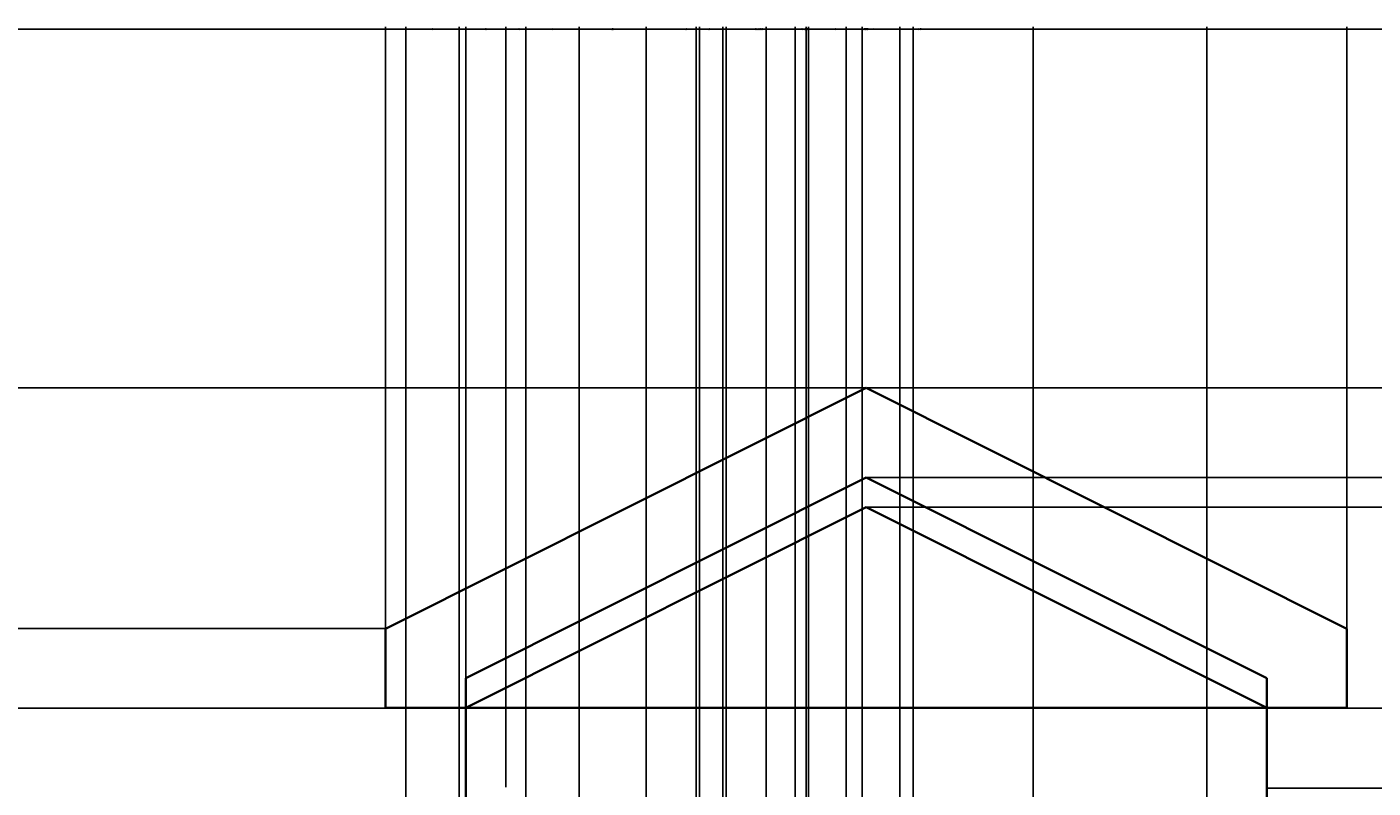
# Model space of a CAD drawing. Units: inches. Extents: x 2154 to 2740, y 571 to 1084.
# Tile 11 of 13: x 2384 to 2485, y 1027 to 1084. Entities that reach past the tile are written whole.
import ezdxf

# ---------------------------------------------------------------- set-up
doc = ezdxf.new("R2010")
doc.units = ezdxf.units.IN
doc.layers.add('A-ANNO-DIMS', color=2, linetype='Continuous', lineweight=18)
doc.layers.add('A-ROOF', color=1, linetype='Continuous', lineweight=35)
doc.styles.get("Standard").update_dxf_attribs({"font": 'arial.ttf'})
doc.dimstyles.get("Standard").update_dxf_attribs({"dimtxt": 0.18, "dimasz": 0.18, "dimexe": 0.18, "dimexo": 0.0625, "dimgap": 0.09, "dimtad": 0, "dimtih": 1, "dimtoh": 1, "dimdec": 4, "dimzin": 0, "dimdsep": 46, "dimtxsty": 'Standard', "dimcen": 0.09, "dimadec": 0, "dimazin": 0, "dimtfac": 1, "dimtdec": 4, "dimtofl": 0, "dimtmove": 0, "dimatfit": 3, "dimfxl": 1, "dimtolj": 1, "dimtzin": 0, "dimarcsym": 0})

# ---------------------------------------------------------------- blocks, each defined once
blk = doc.blocks.new('*D7')
at = {"layer": 'A-ANNO-DIMS', "color": 0, "lineweight": -2, "transparency": 16777216}
for p, q in [((2181.21, 981.59), (2181.21, 1084.04)), ((2181.39, 1083.86), (2446.92, 1083.86)), ((2713.03, 1083.86), (2447.49, 1083.86)), ((2713.21, 981.59), (2713.21, 1084.04))]:
    blk.add_line(p, q, dxfattribs=at)
at = {"layer": 'A-ANNO-DIMS', "color": 0, "transparency": 16777216}
for points in [[(2181.39, 1083.89), (2181.39, 1083.83), (2181.21, 1083.86)], [(2713.03, 1083.89), (2713.03, 1083.83), (2713.21, 1083.86)]]:
    blk.add_solid(points, dxfattribs=at)
at = {"layer": 'Defpoints', "color": 0, "transparency": 16777216}
for p in [(2713.21, 1083.86), (2181.21, 981.53), (2713.21, 981.53)]:
    blk.add_point(p, dxfattribs=at)
at = {"layer": 'A-ANNO-DIMS', "color": 0, "transparency": 16777216, "insert": (2447.21, 1083.86), "char_height": 0.18, "attachment_point": 5}
blk.add_mtext('\\A1;532', dxfattribs=at)
blk = doc.blocks.new('*D10')
at = {"layer": 'A-ANNO-DIMS', "color": 0, "lineweight": -2, "transparency": 16777216}
for p, q in [((2447.14, 1057.01), (2154.18, 1057.01)), ((2154.36, 1056.83), (2154.36, 827.45)), ((2154.36, 597.71), (2154.36, 827.09)), ((2181.14, 597.53), (2154.18, 597.53))]:
    blk.add_line(p, q, dxfattribs=at)
at = {"layer": 'A-ANNO-DIMS', "color": 0, "transparency": 16777216}
for points in [[(2154.33, 1056.83), (2154.39, 1056.83), (2154.36, 1057.01)], [(2154.33, 597.71), (2154.39, 597.71), (2154.36, 597.53)]]:
    blk.add_solid(points, dxfattribs=at)
at = {"layer": 'Defpoints', "color": 0, "transparency": 16777216}
for p in [(2154.36, 1057.01), (2447.21, 1057.01), (2181.21, 597.53)]:
    blk.add_point(p, dxfattribs=at)
at = {"layer": 'A-ANNO-DIMS', "color": 0, "transparency": 16777216, "insert": (2154.36, 827.27), "char_height": 0.18, "attachment_point": 5}
blk.add_mtext('\\A1;459.5', dxfattribs=at)
blk = doc.blocks.new('*D13')
at = {"layer": 'A-ANNO-DIMS', "color": 0, "lineweight": -2, "transparency": 16777216}
for p, q in [((2447.27, 1057.01), (2740.24, 1057.01)), ((2740.06, 1056.83), (2740.06, 1019.45)), ((2740.06, 981.71), (2740.06, 1019.09)), ((2713.27, 981.53), (2740.24, 981.53))]:
    blk.add_line(p, q, dxfattribs=at)
at = {"layer": 'A-ANNO-DIMS', "color": 0, "transparency": 16777216}
for points in [[(2740.03, 1056.83), (2740.09, 1056.83), (2740.06, 1057.01)], [(2740.03, 981.71), (2740.09, 981.71), (2740.06, 981.53)]]:
    blk.add_solid(points, dxfattribs=at)
at = {"layer": 'Defpoints', "color": 0, "transparency": 16777216}
for p in [(2447.21, 1057.01), (2740.06, 1057.01), (2713.21, 981.53)]:
    blk.add_point(p, dxfattribs=at)
at = {"layer": 'A-ANNO-DIMS', "color": 0, "transparency": 16777216, "insert": (2740.06, 1019.27), "char_height": 0.18, "attachment_point": 5}
blk.add_mtext('\\A1;75.47', dxfattribs=at)
blk = doc.blocks.new('*D32')
at = {"layer": 'A-ANNO-DIMS', "color": 0, "lineweight": -2, "transparency": 16777216}
for p, q in [((2412.71, 873.59), (2412.71, 1084.04)), ((2412.89, 1083.86), (2442.49, 1083.86)), ((2472.53, 1083.86), (2442.93, 1083.86)), ((2472.71, 873.59), (2472.71, 1084.04))]:
    blk.add_line(p, q, dxfattribs=at)
at = {"layer": 'A-ANNO-DIMS', "color": 0, "transparency": 16777216}
for points in [[(2412.89, 1083.89), (2412.89, 1083.83), (2412.71, 1083.86)], [(2472.53, 1083.89), (2472.53, 1083.83), (2472.71, 1083.86)]]:
    blk.add_solid(points, dxfattribs=at)
at = {"layer": 'Defpoints', "color": 0, "transparency": 16777216}
for p in [(2472.71, 1083.86), (2412.71, 873.53), (2472.71, 873.53)]:
    blk.add_point(p, dxfattribs=at)
at = {"layer": 'A-ANNO-DIMS', "color": 0, "transparency": 16777216, "insert": (2442.71, 1083.86), "char_height": 0.18, "attachment_point": 5}
blk.add_mtext('\\A1;60', dxfattribs=at)
blk = doc.blocks.new('*D34')
at = {"layer": 'A-ANNO-DIMS', "color": 0, "lineweight": -2, "transparency": 16777216}
for p, q in [((2417.14, 1033.01), (2154.18, 1033.01)), ((2154.36, 1032.83), (2154.36, 1001.96)), ((2154.36, 970.71), (2154.36, 1001.59)), ((2417.14, 970.53), (2154.18, 970.53))]:
    blk.add_line(p, q, dxfattribs=at)
at = {"layer": 'A-ANNO-DIMS', "color": 0, "transparency": 16777216}
for points in [[(2154.33, 1032.83), (2154.39, 1032.83), (2154.36, 1033.01)], [(2154.33, 970.71), (2154.39, 970.71), (2154.36, 970.53)]]:
    blk.add_solid(points, dxfattribs=at)
at = {"layer": 'Defpoints', "color": 0, "transparency": 16777216}
for p in [(2154.36, 1033.01), (2417.21, 1033.01), (2417.21, 970.53)]:
    blk.add_point(p, dxfattribs=at)
at = {"layer": 'A-ANNO-DIMS', "color": 0, "transparency": 16777216, "insert": (2154.36, 1001.77), "char_height": 0.18, "attachment_point": 5}
blk.add_mtext('\\A1;62.48', dxfattribs=at)
blk = doc.blocks.new('*D66')
at = {"layer": 'A-ANNO-DIMS', "color": 0, "lineweight": -2, "transparency": 16777216}
for p, q in [((2411.21, 1033.08), (2411.21, 1084.04)), ((2411.39, 1083.86), (2446.99, 1083.86)), ((2483.03, 1083.86), (2447.42, 1083.86)), ((2483.21, 1033.08), (2483.21, 1084.04))]:
    blk.add_line(p, q, dxfattribs=at)
at = {"layer": 'A-ANNO-DIMS', "color": 0, "transparency": 16777216}
for points in [[(2411.39, 1083.89), (2411.39, 1083.83), (2411.21, 1083.86)], [(2483.03, 1083.89), (2483.03, 1083.83), (2483.21, 1083.86)]]:
    blk.add_solid(points, dxfattribs=at)
at = {"layer": 'Defpoints', "color": 0, "transparency": 16777216}
for p in [(2483.21, 1083.86), (2411.21, 1033.01), (2483.21, 1033.01)]:
    blk.add_point(p, dxfattribs=at)
at = {"layer": 'A-ANNO-DIMS', "color": 0, "transparency": 16777216, "insert": (2447.21, 1083.86), "char_height": 0.18, "attachment_point": 5}
blk.add_mtext('\\A1;72', dxfattribs=at)
blk = doc.blocks.new('*D67')
at = {"layer": 'A-ANNO-DIMS', "color": 0, "lineweight": -2, "transparency": 16777216}
for p, q in [((2411.14, 1038.96), (2154.18, 1038.96)), ((2154.36, 1038.78), (2154.36, 1036.17)), ((2154.36, 1033.19), (2154.36, 1035.8)), ((2411.14, 1033.01), (2154.18, 1033.01))]:
    blk.add_line(p, q, dxfattribs=at)
at = {"layer": 'A-ANNO-DIMS', "color": 0, "transparency": 16777216}
for points in [[(2154.33, 1038.78), (2154.39, 1038.78), (2154.36, 1038.96)], [(2154.33, 1033.19), (2154.39, 1033.19), (2154.36, 1033.01)]]:
    blk.add_solid(points, dxfattribs=at)
at = {"layer": 'Defpoints', "color": 0, "transparency": 16777216}
for p in [(2154.36, 1038.96), (2411.21, 1038.96), (2411.21, 1033.01)]:
    blk.add_point(p, dxfattribs=at)
at = {"layer": 'A-ANNO-DIMS', "color": 0, "transparency": 16777216, "insert": (2154.36, 1035.99), "char_height": 0.18, "attachment_point": 5}
blk.add_mtext('\\A1;5.941', dxfattribs=at)
blk = doc.blocks.new('*D68')
at = {"layer": 'A-ANNO-DIMS', "color": 0, "lineweight": -2, "transparency": 16777216}
for p, q in [((2447.14, 1057.01), (2154.18, 1057.01)), ((2154.36, 1056.83), (2154.36, 1048.16)), ((2154.36, 1039.14), (2154.36, 1047.8)), ((2411.14, 1038.96), (2154.18, 1038.96))]:
    blk.add_line(p, q, dxfattribs=at)
at = {"layer": 'A-ANNO-DIMS', "color": 0, "transparency": 16777216}
for points in [[(2154.33, 1056.83), (2154.39, 1056.83), (2154.36, 1057.01)], [(2154.33, 1039.14), (2154.39, 1039.14), (2154.36, 1038.96)]]:
    blk.add_solid(points, dxfattribs=at)
at = {"layer": 'Defpoints', "color": 0, "transparency": 16777216}
for p in [(2154.36, 1057.01), (2447.21, 1057.01), (2411.21, 1038.96)]:
    blk.add_point(p, dxfattribs=at)
at = {"layer": 'A-ANNO-DIMS', "color": 0, "transparency": 16777216, "insert": (2154.36, 1047.98), "char_height": 0.18, "attachment_point": 5}
blk.add_mtext('\\A1;18.05', dxfattribs=at)
blk = doc.blocks.new('*D69')
at = {"layer": 'A-ANNO-DIMS', "color": 0, "lineweight": -2, "transparency": 16777216}
for p, q in [((2447.27, 1057.01), (2740.24, 1057.01)), ((2740.06, 1056.83), (2740.06, 1053.83)), ((2740.06, 1050.47), (2740.06, 1053.47)), ((2447.27, 1050.29), (2740.24, 1050.29))]:
    blk.add_line(p, q, dxfattribs=at)
at = {"layer": 'A-ANNO-DIMS', "color": 0, "transparency": 16777216}
for points in [[(2740.03, 1056.83), (2740.09, 1056.83), (2740.06, 1057.01)], [(2740.03, 1050.47), (2740.09, 1050.47), (2740.06, 1050.29)]]:
    blk.add_solid(points, dxfattribs=at)
at = {"layer": 'Defpoints', "color": 0, "transparency": 16777216}
for p in [(2447.21, 1057.01), (2740.06, 1057.01), (2447.21, 1050.29)]:
    blk.add_point(p, dxfattribs=at)
at = {"layer": 'A-ANNO-DIMS', "color": 0, "transparency": 16777216, "insert": (2740.06, 1053.65), "char_height": 0.18, "attachment_point": 5}
blk.add_mtext('\\A1;6.712', dxfattribs=at)
blk = doc.blocks.new('*D70')
at = {"layer": 'A-ANNO-DIMS', "color": 0, "lineweight": -2, "transparency": 16777216}
for p, q in [((2447.27, 1050.29), (2740.24, 1050.29)), ((2740.06, 1050.11), (2740.06, 1049.36)), ((2740.06, 1048.24), (2740.06, 1048.99)), ((2447.27, 1048.06), (2740.24, 1048.06))]:
    blk.add_line(p, q, dxfattribs=at)
at = {"layer": 'A-ANNO-DIMS', "color": 0, "transparency": 16777216}
for points in [[(2740.03, 1050.11), (2740.09, 1050.11), (2740.06, 1050.29)], [(2740.03, 1048.24), (2740.09, 1048.24), (2740.06, 1048.06)]]:
    blk.add_solid(points, dxfattribs=at)
at = {"layer": 'Defpoints', "color": 0, "transparency": 16777216}
for p in [(2447.21, 1050.29), (2740.06, 1050.29), (2447.21, 1048.06)]:
    blk.add_point(p, dxfattribs=at)
at = {"layer": 'A-ANNO-DIMS', "color": 0, "transparency": 16777216, "insert": (2740.06, 1049.17), "char_height": 0.18, "attachment_point": 5}
blk.add_mtext('\\A1;2.24', dxfattribs=at)
blk = doc.blocks.new('*D71')
at = {"layer": 'A-ANNO-DIMS', "color": 0, "lineweight": -2, "transparency": 16777216}
for p, q in [((2477.27, 1033.01), (2740.24, 1033.01)), ((2740.06, 1032.83), (2740.06, 1030.2)), ((2740.06, 1027.19), (2740.06, 1029.83)), ((2477.27, 1027.01), (2740.24, 1027.01))]:
    blk.add_line(p, q, dxfattribs=at)
at = {"layer": 'A-ANNO-DIMS', "color": 0, "transparency": 16777216}
for points in [[(2740.03, 1032.83), (2740.09, 1032.83), (2740.06, 1033.01)], [(2740.03, 1027.19), (2740.09, 1027.19), (2740.06, 1027.01)]]:
    blk.add_solid(points, dxfattribs=at)
at = {"layer": 'Defpoints', "color": 0, "transparency": 16777216}
for p in [(2477.21, 1033.01), (2740.06, 1033.01), (2477.21, 1027.01)]:
    blk.add_point(p, dxfattribs=at)
at = {"layer": 'A-ANNO-DIMS', "color": 0, "transparency": 16777216, "insert": (2740.06, 1030.01), "char_height": 0.18, "attachment_point": 5}
blk.add_mtext('\\A1;6', dxfattribs=at)
blk = doc.blocks.new('*D72')
at = {"layer": 'A-ANNO-DIMS', "color": 0, "lineweight": -2, "transparency": 16777216}
for p, q in [((2477.27, 1027.01), (2740.24, 1027.01)), ((2740.06, 1026.83), (2740.06, 1001.96)), ((2740.06, 976.71), (2740.06, 1001.59)), ((2477.27, 976.53), (2740.24, 976.53))]:
    blk.add_line(p, q, dxfattribs=at)
at = {"layer": 'A-ANNO-DIMS', "color": 0, "transparency": 16777216}
for points in [[(2740.03, 1026.83), (2740.09, 1026.83), (2740.06, 1027.01)], [(2740.03, 976.71), (2740.09, 976.71), (2740.06, 976.53)]]:
    blk.add_solid(points, dxfattribs=at)
at = {"layer": 'Defpoints', "color": 0, "transparency": 16777216}
for p in [(2477.21, 1027.01), (2740.06, 1027.01), (2477.21, 976.53)]:
    blk.add_point(p, dxfattribs=at)
at = {"layer": 'A-ANNO-DIMS', "color": 0, "transparency": 16777216, "insert": (2740.06, 1001.77), "char_height": 0.18, "attachment_point": 5}
blk.add_mtext('\\A1;50.48', dxfattribs=at)
blk = doc.blocks.new('*D74')
at = {"layer": 'A-ANNO-DIMS', "color": 0, "lineweight": -2, "transparency": 16777216}
for p, q in [((2417.21, 1027.08), (2417.21, 1084.04)), ((2417.39, 1083.86), (2418.56, 1083.86)), ((2420.03, 1083.86), (2418.86, 1083.86)), ((2420.21, 1027.08), (2420.21, 1084.04))]:
    blk.add_line(p, q, dxfattribs=at)
at = {"layer": 'A-ANNO-DIMS', "color": 0, "transparency": 16777216}
for points in [[(2417.39, 1083.89), (2417.39, 1083.83), (2417.21, 1083.86)], [(2420.03, 1083.89), (2420.03, 1083.83), (2420.21, 1083.86)]]:
    blk.add_solid(points, dxfattribs=at)
at = {"layer": 'Defpoints', "color": 0, "transparency": 16777216}
for p in [(2420.21, 1083.86), (2417.21, 1027.01), (2420.21, 1027.01)]:
    blk.add_point(p, dxfattribs=at)
at = {"layer": 'A-ANNO-DIMS', "color": 0, "transparency": 16777216, "insert": (2418.71, 1083.86), "char_height": 0.18, "attachment_point": 5}
blk.add_mtext('\\A1;3', dxfattribs=at)
blk = doc.blocks.new('*D79')
at = {"layer": 'A-ANNO-DIMS', "color": 0, "lineweight": -2, "transparency": 16777216}
for p, q in [((2436.46, 1010.97), (2436.46, 1084.04)), ((2436.64, 1083.86), (2438.78, 1083.86)), ((2441.71, 1083.86), (2439.57, 1083.86)), ((2441.89, 1010.97), (2441.89, 1084.04))]:
    blk.add_line(p, q, dxfattribs=at)
at = {"layer": 'A-ANNO-DIMS', "color": 0, "transparency": 16777216}
for points in [[(2436.64, 1083.89), (2436.64, 1083.83), (2436.46, 1083.86)], [(2441.71, 1083.89), (2441.71, 1083.83), (2441.89, 1083.86)]]:
    blk.add_solid(points, dxfattribs=at)
at = {"layer": 'Defpoints', "color": 0, "transparency": 16777216}
for p in [(2441.89, 1083.86), (2436.46, 1010.91), (2441.89, 1010.91)]:
    blk.add_point(p, dxfattribs=at)
at = {"layer": 'A-ANNO-DIMS', "color": 0, "transparency": 16777216, "insert": (2439.17, 1083.86), "char_height": 0.18, "attachment_point": 5}
blk.add_mtext('\\A1;5.433', dxfattribs=at)
blk = doc.blocks.new('*D80')
at = {"layer": 'A-ANNO-DIMS', "color": 0, "lineweight": -2, "transparency": 16777216}
for p, q in [((2441.89, 1010.97), (2441.89, 1084.04)), ((2442.07, 1083.86), (2442.27, 1083.86)), ((2442.71, 1083.86), (2442.51, 1083.86)), ((2442.89, 1010.97), (2442.89, 1084.04))]:
    blk.add_line(p, q, dxfattribs=at)
at = {"layer": 'A-ANNO-DIMS', "color": 0, "transparency": 16777216}
for points in [[(2442.07, 1083.89), (2442.07, 1083.83), (2441.89, 1083.86)], [(2442.71, 1083.89), (2442.71, 1083.83), (2442.89, 1083.86)]]:
    blk.add_solid(points, dxfattribs=at)
at = {"layer": 'Defpoints', "color": 0, "transparency": 16777216}
for p in [(2442.89, 1083.86), (2441.89, 1010.91), (2442.89, 1010.91)]:
    blk.add_point(p, dxfattribs=at)
at = {"layer": 'A-ANNO-DIMS', "color": 0, "transparency": 16777216, "insert": (2442.39, 1083.86), "char_height": 0.18, "attachment_point": 5}
blk.add_mtext('\\A1;1', dxfattribs=at)
blk = doc.blocks.new('*D81')
at = {"layer": 'A-ANNO-DIMS', "color": 0, "lineweight": -2, "transparency": 16777216}
for p, q in [((2442.89, 1010.97), (2442.89, 1084.04)), ((2443.07, 1083.86), (2444.74, 1083.86)), ((2446.71, 1083.86), (2445.04, 1083.86)), ((2446.89, 1010.97), (2446.89, 1084.04))]:
    blk.add_line(p, q, dxfattribs=at)
at = {"layer": 'A-ANNO-DIMS', "color": 0, "transparency": 16777216}
for points in [[(2443.07, 1083.89), (2443.07, 1083.83), (2442.89, 1083.86)], [(2446.71, 1083.89), (2446.71, 1083.83), (2446.89, 1083.86)]]:
    blk.add_solid(points, dxfattribs=at)
at = {"layer": 'Defpoints', "color": 0, "transparency": 16777216}
for p in [(2446.89, 1083.86), (2442.89, 1010.91), (2446.89, 1010.91)]:
    blk.add_point(p, dxfattribs=at)
at = {"layer": 'A-ANNO-DIMS', "color": 0, "transparency": 16777216, "insert": (2444.89, 1083.86), "char_height": 0.18, "attachment_point": 5}
blk.add_mtext('\\A1;4', dxfattribs=at)
blk = doc.blocks.new('*D82')
at = {"layer": 'A-ANNO-DIMS', "color": 0, "lineweight": -2, "transparency": 16777216}
for p, q in [((2434.46, 1012.97), (2434.46, 1084.04)), ((2434.64, 1083.86), (2435.31, 1083.86)), ((2436.28, 1083.86), (2435.61, 1083.86)), ((2436.46, 1010.97), (2436.46, 1084.04))]:
    blk.add_line(p, q, dxfattribs=at)
at = {"layer": 'A-ANNO-DIMS', "color": 0, "transparency": 16777216}
for points in [[(2434.64, 1083.89), (2434.64, 1083.83), (2434.46, 1083.86)], [(2436.28, 1083.89), (2436.28, 1083.83), (2436.46, 1083.86)]]:
    blk.add_solid(points, dxfattribs=at)
at = {"layer": 'Defpoints', "color": 0, "transparency": 16777216}
for p in [(2436.46, 1083.86), (2434.46, 1012.91), (2436.46, 1010.91)]:
    blk.add_point(p, dxfattribs=at)
at = {"layer": 'A-ANNO-DIMS', "color": 0, "transparency": 16777216, "insert": (2435.46, 1083.86), "char_height": 0.18, "attachment_point": 5}
blk.add_mtext('\\A1;2', dxfattribs=at)
blk = doc.blocks.new('*D87')
at = {"layer": 'A-ANNO-DIMS', "color": 0, "lineweight": -2, "transparency": 16777216}
for p, q in [((2421.71, 725.29), (2421.71, 1084.04)), ((2421.89, 1083.86), (2423.55, 1083.86)), ((2425.53, 1083.86), (2423.86, 1083.86)), ((2425.71, 721.29), (2425.71, 1084.04))]:
    blk.add_line(p, q, dxfattribs=at)
at = {"layer": 'A-ANNO-DIMS', "color": 0, "transparency": 16777216}
for points in [[(2421.89, 1083.89), (2421.89, 1083.83), (2421.71, 1083.86)], [(2425.53, 1083.89), (2425.53, 1083.83), (2425.71, 1083.86)]]:
    blk.add_solid(points, dxfattribs=at)
at = {"layer": 'Defpoints', "color": 0, "transparency": 16777216}
for p in [(2425.71, 1083.86), (2421.71, 725.23), (2425.71, 721.23)]:
    blk.add_point(p, dxfattribs=at)
at = {"layer": 'A-ANNO-DIMS', "color": 0, "transparency": 16777216, "insert": (2423.71, 1083.86), "char_height": 0.18, "attachment_point": 5}
blk.add_mtext('\\A1;4', dxfattribs=at)
blk = doc.blocks.new('*D90')
at = {"layer": 'A-ANNO-DIMS', "color": 0, "lineweight": -2, "transparency": 16777216}
for p, q in [((2434.71, 712.29), (2434.71, 1084.04)), ((2434.89, 1083.86), (2442.5, 1083.86)), ((2450.53, 1083.86), (2442.92, 1083.86)), ((2450.71, 712.29), (2450.71, 1084.04))]:
    blk.add_line(p, q, dxfattribs=at)
at = {"layer": 'A-ANNO-DIMS', "color": 0, "transparency": 16777216}
for points in [[(2434.89, 1083.89), (2434.89, 1083.83), (2434.71, 1083.86)], [(2450.53, 1083.89), (2450.53, 1083.83), (2450.71, 1083.86)]]:
    blk.add_solid(points, dxfattribs=at)
at = {"layer": 'Defpoints', "color": 0, "transparency": 16777216}
for p in [(2450.71, 1083.86), (2434.71, 712.23), (2450.71, 712.23)]:
    blk.add_point(p, dxfattribs=at)
at = {"layer": 'A-ANNO-DIMS', "color": 0, "transparency": 16777216, "insert": (2442.71, 1083.86), "char_height": 0.18, "attachment_point": 5}
blk.add_mtext('\\A1;16', dxfattribs=at)
blk = doc.blocks.new('*D93')
at = {"layer": 'A-ANNO-DIMS', "color": 0, "lineweight": -2, "transparency": 16777216}
for p, q in [((2439.71, 703.29), (2439.71, 1084.04)), ((2439.89, 1083.86), (2442.56, 1083.86)), ((2445.53, 1083.86), (2442.86, 1083.86)), ((2445.71, 703.29), (2445.71, 1084.04))]:
    blk.add_line(p, q, dxfattribs=at)
at = {"layer": 'A-ANNO-DIMS', "color": 0, "transparency": 16777216}
for points in [[(2439.89, 1083.89), (2439.89, 1083.83), (2439.71, 1083.86)], [(2445.53, 1083.89), (2445.53, 1083.83), (2445.71, 1083.86)]]:
    blk.add_solid(points, dxfattribs=at)
at = {"layer": 'Defpoints', "color": 0, "transparency": 16777216}
for p in [(2445.71, 1083.86), (2439.71, 703.23), (2445.71, 703.23)]:
    blk.add_point(p, dxfattribs=at)
at = {"layer": 'A-ANNO-DIMS', "color": 0, "transparency": 16777216, "insert": (2442.71, 1083.86), "char_height": 0.18, "attachment_point": 5}
blk.add_mtext('\\A1;6', dxfattribs=at)
blk = doc.blocks.new('*D94')
at = {"layer": 'A-ANNO-DIMS', "color": 0, "lineweight": -2, "transparency": 16777216}
for p, q in [((2445.71, 703.29), (2445.71, 1084.04)), ((2445.89, 1083.86), (2447.55, 1083.86)), ((2449.53, 1083.86), (2447.86, 1083.86)), ((2449.71, 703.29), (2449.71, 1084.04))]:
    blk.add_line(p, q, dxfattribs=at)
at = {"layer": 'A-ANNO-DIMS', "color": 0, "transparency": 16777216}
for points in [[(2445.89, 1083.89), (2445.89, 1083.83), (2445.71, 1083.86)], [(2449.53, 1083.89), (2449.53, 1083.83), (2449.71, 1083.86)]]:
    blk.add_solid(points, dxfattribs=at)
at = {"layer": 'Defpoints', "color": 0, "transparency": 16777216}
for p in [(2449.71, 1083.86), (2445.71, 703.23), (2449.71, 703.23)]:
    blk.add_point(p, dxfattribs=at)
at = {"layer": 'A-ANNO-DIMS', "color": 0, "transparency": 16777216, "insert": (2447.71, 1083.86), "char_height": 0.18, "attachment_point": 5}
blk.add_mtext('\\A1;4', dxfattribs=at)
blk = doc.blocks.new('*D99')
at = {"layer": 'A-ANNO-DIMS', "color": 0, "lineweight": -2, "transparency": 16777216}
for p, q in [((2412.71, 873.59), (2412.71, 1084.04)), ((2412.89, 1083.86), (2414.55, 1083.86)), ((2416.53, 1083.86), (2414.86, 1083.86)), ((2416.71, 869.59), (2416.71, 1084.04))]:
    blk.add_line(p, q, dxfattribs=at)
at = {"layer": 'A-ANNO-DIMS', "color": 0, "transparency": 16777216}
for points in [[(2412.89, 1083.89), (2412.89, 1083.83), (2412.71, 1083.86)], [(2416.53, 1083.89), (2416.53, 1083.83), (2416.71, 1083.86)]]:
    blk.add_solid(points, dxfattribs=at)
at = {"layer": 'Defpoints', "color": 0, "transparency": 16777216}
for p in [(2416.71, 1083.86), (2412.71, 873.53), (2416.71, 869.53)]:
    blk.add_point(p, dxfattribs=at)
at = {"layer": 'A-ANNO-DIMS', "color": 0, "transparency": 16777216, "insert": (2414.71, 1083.86), "char_height": 0.18, "attachment_point": 5}
blk.add_mtext('\\A1;4', dxfattribs=at)
blk = doc.blocks.new('*D101')
at = {"layer": 'A-ANNO-DIMS', "color": 0, "lineweight": -2, "transparency": 16777216}
for p, q in [((2416.71, 869.59), (2416.71, 1084.04)), ((2416.89, 1083.86), (2421.06, 1083.86)), ((2425.53, 1083.86), (2421.36, 1083.86)), ((2425.71, 860.59), (2425.71, 1084.04))]:
    blk.add_line(p, q, dxfattribs=at)
at = {"layer": 'A-ANNO-DIMS', "color": 0, "transparency": 16777216}
for points in [[(2416.89, 1083.89), (2416.89, 1083.83), (2416.71, 1083.86)], [(2425.53, 1083.89), (2425.53, 1083.83), (2425.71, 1083.86)]]:
    blk.add_solid(points, dxfattribs=at)
at = {"layer": 'Defpoints', "color": 0, "transparency": 16777216}
for p in [(2425.71, 1083.86), (2416.71, 869.53), (2425.71, 860.53)]:
    blk.add_point(p, dxfattribs=at)
at = {"layer": 'A-ANNO-DIMS', "color": 0, "transparency": 16777216, "insert": (2421.21, 1083.86), "char_height": 0.18, "attachment_point": 5}
blk.add_mtext('\\A1;9', dxfattribs=at)
blk = doc.blocks.new('*D102')
at = {"layer": 'A-ANNO-DIMS', "color": 0, "lineweight": -2, "transparency": 16777216}
for p, q in [((2425.71, 860.59), (2425.71, 1084.04)), ((2425.89, 1083.86), (2428.06, 1083.86)), ((2430.53, 1083.86), (2428.36, 1083.86)), ((2430.71, 860.59), (2430.71, 1084.04))]:
    blk.add_line(p, q, dxfattribs=at)
at = {"layer": 'A-ANNO-DIMS', "color": 0, "transparency": 16777216}
for points in [[(2425.89, 1083.89), (2425.89, 1083.83), (2425.71, 1083.86)], [(2430.53, 1083.89), (2430.53, 1083.83), (2430.71, 1083.86)]]:
    blk.add_solid(points, dxfattribs=at)
at = {"layer": 'Defpoints', "color": 0, "transparency": 16777216}
for p in [(2430.71, 1083.86), (2425.71, 860.53), (2430.71, 860.53)]:
    blk.add_point(p, dxfattribs=at)
at = {"layer": 'A-ANNO-DIMS', "color": 0, "transparency": 16777216, "insert": (2428.21, 1083.86), "char_height": 0.18, "attachment_point": 5}
blk.add_mtext('\\A1;5', dxfattribs=at)
blk = doc.blocks.new('*D103')
at = {"layer": 'A-ANNO-DIMS', "color": 0, "lineweight": -2, "transparency": 16777216}
for p, q in [((2430.71, 860.59), (2430.71, 1084.04)), ((2430.89, 1083.86), (2433.56, 1083.86)), ((2436.53, 1083.86), (2433.86, 1083.86)), ((2436.71, 860.59), (2436.71, 1084.04))]:
    blk.add_line(p, q, dxfattribs=at)
at = {"layer": 'A-ANNO-DIMS', "color": 0, "transparency": 16777216}
for points in [[(2430.89, 1083.89), (2430.89, 1083.83), (2430.71, 1083.86)], [(2436.53, 1083.89), (2436.53, 1083.83), (2436.71, 1083.86)]]:
    blk.add_solid(points, dxfattribs=at)
at = {"layer": 'Defpoints', "color": 0, "transparency": 16777216}
for p in [(2436.71, 1083.86), (2430.71, 860.53), (2436.71, 860.53)]:
    blk.add_point(p, dxfattribs=at)
at = {"layer": 'A-ANNO-DIMS', "color": 0, "transparency": 16777216, "insert": (2433.71, 1083.86), "char_height": 0.18, "attachment_point": 5}
blk.add_mtext('\\A1;6', dxfattribs=at)
blk = doc.blocks.new('*D104')
at = {"layer": 'A-ANNO-DIMS', "color": 0, "lineweight": -2, "transparency": 16777216}
for p, q in [((2436.71, 860.59), (2436.71, 1084.04)), ((2436.89, 1083.86), (2439.56, 1083.86)), ((2442.53, 1083.86), (2439.86, 1083.86)), ((2442.71, 860.59), (2442.71, 1084.04))]:
    blk.add_line(p, q, dxfattribs=at)
at = {"layer": 'A-ANNO-DIMS', "color": 0, "transparency": 16777216}
for points in [[(2436.89, 1083.89), (2436.89, 1083.83), (2436.71, 1083.86)], [(2442.53, 1083.89), (2442.53, 1083.83), (2442.71, 1083.86)]]:
    blk.add_solid(points, dxfattribs=at)
at = {"layer": 'Defpoints', "color": 0, "transparency": 16777216}
for p in [(2442.71, 1083.86), (2436.71, 860.53), (2442.71, 860.53)]:
    blk.add_point(p, dxfattribs=at)
at = {"layer": 'A-ANNO-DIMS', "color": 0, "transparency": 16777216, "insert": (2439.71, 1083.86), "char_height": 0.18, "attachment_point": 5}
blk.add_mtext('\\A1;6', dxfattribs=at)
blk = doc.blocks.new('*D105')
at = {"layer": 'A-ANNO-DIMS', "color": 0, "lineweight": -2, "transparency": 16777216}
for p, q in [((2442.71, 860.59), (2442.71, 1084.04)), ((2442.89, 1083.86), (2451, 1083.86)), ((2459.53, 1083.86), (2451.42, 1083.86)), ((2459.71, 860.59), (2459.71, 1084.04))]:
    blk.add_line(p, q, dxfattribs=at)
at = {"layer": 'A-ANNO-DIMS', "color": 0, "transparency": 16777216}
for points in [[(2442.89, 1083.89), (2442.89, 1083.83), (2442.71, 1083.86)], [(2459.53, 1083.89), (2459.53, 1083.83), (2459.71, 1083.86)]]:
    blk.add_solid(points, dxfattribs=at)
at = {"layer": 'Defpoints', "color": 0, "transparency": 16777216}
for p in [(2459.71, 1083.86), (2442.71, 860.53), (2459.71, 860.53)]:
    blk.add_point(p, dxfattribs=at)
at = {"layer": 'A-ANNO-DIMS', "color": 0, "transparency": 16777216, "insert": (2451.21, 1083.86), "char_height": 0.18, "attachment_point": 5}
blk.add_mtext('\\A1;17', dxfattribs=at)

msp = doc.modelspace()

# ---------------------------------------------------------------- linework, layer by layer
at = {"layer": 'A-ROOF'}
for p, q in [((2411.2067, 1038.9557), (2447.2067, 1057.0053)), ((2447.2067, 1057.0053), (2483.2067, 1038.9557)), ((2417.2067, 1035.2521), (2447.2067, 1050.2934)), ((2447.2067, 1050.2934), (2477.2067, 1035.2521)), ((2417.2067, 1033.0148), (2447.2067, 1048.0561)), ((2447.2067, 1048.0561), (2477.2067, 1033.0148)), ((2411.2067, 1035.2521), (2411.2067, 1038.9557)), ((2483.2067, 1035.2521), (2483.2067, 1038.9557)), ((2411.2067, 1033.0148), (2411.2067, 1035.2521)), ((2417.2067, 970.5321), (2417.2067, 1035.2521)), ((2477.2067, 970.5321), (2477.2067, 1035.2521)), ((2483.2067, 1033.0148), (2483.2067, 1035.2521)), ((2411.2067, 1033.0148), (2483.2067, 1033.0148))]:
    msp.add_line(p, q, dxfattribs=at)

# ---------------------------------------------------------------- dimensions: what is measured, and where the dimension line sits
at = {"layer": 'A-ANNO-DIMS'}
for base, p1, p2, override, picture, middle in [((2713.2067, 1083.8553), (2181.2067, 981.5321), (2713.2067, 981.5321), {"dimdec": 0, "dimlfac": 1, "dimrnd": 0, "dimzin": 0, "dimdsep": 46, "dimlunit": 2}, '*D7', (2447.2067, 1083.8553)), ((2483.2067, 1083.8553), (2411.2067, 1033.0148), (2483.2067, 1033.0148), {"dimdec": 0, "dimlfac": 1, "dimrnd": 0, "dimzin": 0, "dimdsep": 46, "dimlunit": 2}, '*D66', (2447.2067, 1083.8553)), ((2472.7067, 1083.8553), (2412.7067, 873.5321), (2472.7067, 873.5321), {"dimdec": 0, "dimlfac": 1, "dimrnd": 0, "dimzin": 0, "dimdsep": 46, "dimlunit": 2}, '*D32', (2442.7067, 1083.8553)), ((2416.7067, 1083.8553), (2412.7067, 873.5321), (2416.7067, 869.5321), {"dimdec": 0, "dimlfac": 1, "dimrnd": 0, "dimzin": 0, "dimdsep": 46, "dimlunit": 2}, '*D99', (2414.7067, 1083.8553)), ((2425.7067, 1083.8553), (2416.7067, 869.5321), (2425.7067, 860.5321), {"dimdec": 0, "dimlfac": 1, "dimrnd": 0, "dimzin": 0, "dimdsep": 46, "dimlunit": 2}, '*D101', (2421.2067, 1083.8553)), ((2420.2067, 1083.8553), (2417.2067, 1027.0148), (2420.2067, 1027.0148), {"dimdec": 0, "dimlfac": 1, "dimrnd": 0, "dimzin": 0, "dimdsep": 46, "dimlunit": 2}, '*D74', (2418.7067, 1083.8553)), ((2425.7067, 1083.8553), (2421.7067, 725.2281), (2425.7067, 721.2281), {"dimdec": 0, "dimlfac": 1, "dimrnd": 0, "dimzin": 0, "dimdsep": 46, "dimlunit": 2}, '*D87', (2423.7067, 1083.8553)), ((2430.7067, 1083.8553), (2425.7067, 860.5321), (2430.7067, 860.5321), {"dimdec": 0, "dimlfac": 1, "dimrnd": 0, "dimzin": 0, "dimdsep": 46, "dimlunit": 2}, '*D102', (2428.2067, 1083.8553)), ((2436.7067, 1083.8553), (2430.7067, 860.5321), (2436.7067, 860.5321), {"dimdec": 0, "dimlfac": 1, "dimrnd": 0, "dimzin": 0, "dimdsep": 46, "dimlunit": 2}, '*D103', (2433.7067, 1083.8553)), ((2436.4565, 1083.8553), (2434.4565, 1012.9076), (2436.4565, 1010.9076), {"dimdec": 0, "dimlfac": 1, "dimrnd": 0, "dimzin": 0, "dimdsep": 46, "dimlunit": 2}, '*D82', (2435.4565, 1083.8553)), ((2450.7067, 1083.8553), (2434.7067, 712.2281), (2450.7067, 712.2281), {"dimdec": 0, "dimlfac": 1, "dimrnd": 0, "dimzin": 0, "dimdsep": 46, "dimlunit": 2}, '*D90', (2442.7067, 1083.8553)), ((2441.8896, 1083.8553), (2436.4565, 1010.9076), (2441.8896, 1010.9076), {"dimdec": 3, "dimlfac": 1, "dimrnd": 0, "dimzin": 0, "dimdsep": 46, "dimlunit": 2}, '*D79', (2439.173, 1083.8553)), ((2442.7067, 1083.8553), (2436.7067, 860.5321), (2442.7067, 860.5321), {"dimdec": 0, "dimlfac": 1, "dimrnd": 0, "dimzin": 0, "dimdsep": 46, "dimlunit": 2}, '*D104', (2439.7067, 1083.8553)), ((2445.7067, 1083.8553), (2439.7067, 703.2281), (2445.7067, 703.2281), {"dimdec": 0, "dimlfac": 1, "dimrnd": 0, "dimzin": 0, "dimdsep": 46, "dimlunit": 2}, '*D93', (2442.7067, 1083.8553)), ((2442.8896, 1083.8553), (2441.8896, 1010.9076), (2442.8896, 1010.9076), {"dimdec": 0, "dimlfac": 1, "dimrnd": 0, "dimzin": 0, "dimdsep": 46, "dimlunit": 2}, '*D80', (2442.3896, 1083.8553)), ((2459.7067, 1083.8553), (2442.7067, 860.5321), (2459.7067, 860.5321), {"dimdec": 0, "dimlfac": 1, "dimrnd": 0, "dimzin": 0, "dimdsep": 46, "dimlunit": 2}, '*D105', (2451.2067, 1083.8553)), ((2446.8896, 1083.8553), (2442.8896, 1010.9076), (2446.8896, 1010.9076), {"dimdec": 0, "dimlfac": 1, "dimrnd": 0, "dimzin": 0, "dimdsep": 46, "dimlunit": 2}, '*D81', (2444.8896, 1083.8553)), ((2449.7067, 1083.8553), (2445.7067, 703.2281), (2449.7067, 703.2281), {"dimdec": 0, "dimlfac": 1, "dimrnd": 0, "dimzin": 0, "dimdsep": 46, "dimlunit": 2}, '*D94', (2447.7067, 1083.8553))]:
    dim = msp.add_linear_dim(base=base, p1=p1, p2=p2, dimstyle='Standard', override=override, dxfattribs=at)
    dim.commit()
    dim.dimension.update_dxf_attribs({"geometry": picture, "text_midpoint": middle})
for base, p1, p2, override, picture, middle in [((2154.3567, 1057.0053), (2181.2067, 597.5321), (2447.2067, 1057.0053), {"dimdec": 1, "dimlfac": 1, "dimrnd": 0, "dimzin": 0, "dimdsep": 46, "dimlunit": 2}, '*D10', (2154.3567, 827.2687)), ((2154.3567, 1057.0053), (2411.2067, 1038.9557), (2447.2067, 1057.0053), {"dimdec": 2, "dimlfac": 1, "dimrnd": 0, "dimzin": 0, "dimdsep": 46, "dimlunit": 2}, '*D68', (2154.3567, 1047.9805)), ((2740.0567, 1057.0053), (2713.2067, 981.5321), (2447.2067, 1057.0053), {"dimdec": 2, "dimlfac": 1, "dimrnd": 0, "dimzin": 0, "dimdsep": 46, "dimlunit": 2}, '*D13', (2740.0567, 1019.2687)), ((2740.0567, 1057.0053), (2447.2067, 1050.2934), (2447.2067, 1057.0053), {"dimdec": 3, "dimlfac": 1, "dimrnd": 0, "dimzin": 0, "dimdsep": 46, "dimlunit": 2}, '*D69', (2740.0567, 1053.6493)), ((2740.0567, 1050.2934), (2447.2067, 1048.0561), (2447.2067, 1050.2934), {"dimdec": 2, "dimlfac": 1, "dimrnd": 0, "dimzin": 0, "dimdsep": 46, "dimlunit": 2}, '*D70', (2740.0567, 1049.1747)), ((2154.3567, 1038.9557), (2411.2067, 1033.0148), (2411.2067, 1038.9557), {"dimdec": 3, "dimlfac": 1, "dimrnd": 0, "dimzin": 0, "dimdsep": 46, "dimlunit": 2}, '*D67', (2154.3567, 1035.9852)), ((2154.3567, 1033.0148), (2417.2067, 970.5321), (2417.2067, 1033.0148), {"dimdec": 2, "dimlfac": 1, "dimrnd": 0, "dimzin": 0, "dimdsep": 46, "dimlunit": 2}, '*D34', (2154.3567, 1001.7734)), ((2740.0567, 1033.0148), (2477.2067, 1027.0148), (2477.2067, 1033.0148), {"dimdec": 0, "dimlfac": 1, "dimrnd": 0, "dimzin": 0, "dimdsep": 46, "dimlunit": 2}, '*D71', (2740.0567, 1030.0148)), ((2740.0567, 1027.0148), (2477.2067, 976.5321), (2477.2067, 1027.0148), {"dimdec": 2, "dimlfac": 1, "dimrnd": 0, "dimzin": 0, "dimdsep": 46, "dimlunit": 2}, '*D72', (2740.0567, 1001.7734))]:
    dim = msp.add_linear_dim(base=base, p1=p1, p2=p2, angle=90, dimstyle='Standard', override=override, dxfattribs=at)
    dim.commit()
    dim.dimension.update_dxf_attribs({"geometry": picture, "text_midpoint": middle})

doc.saveas('drawing.dxf')
